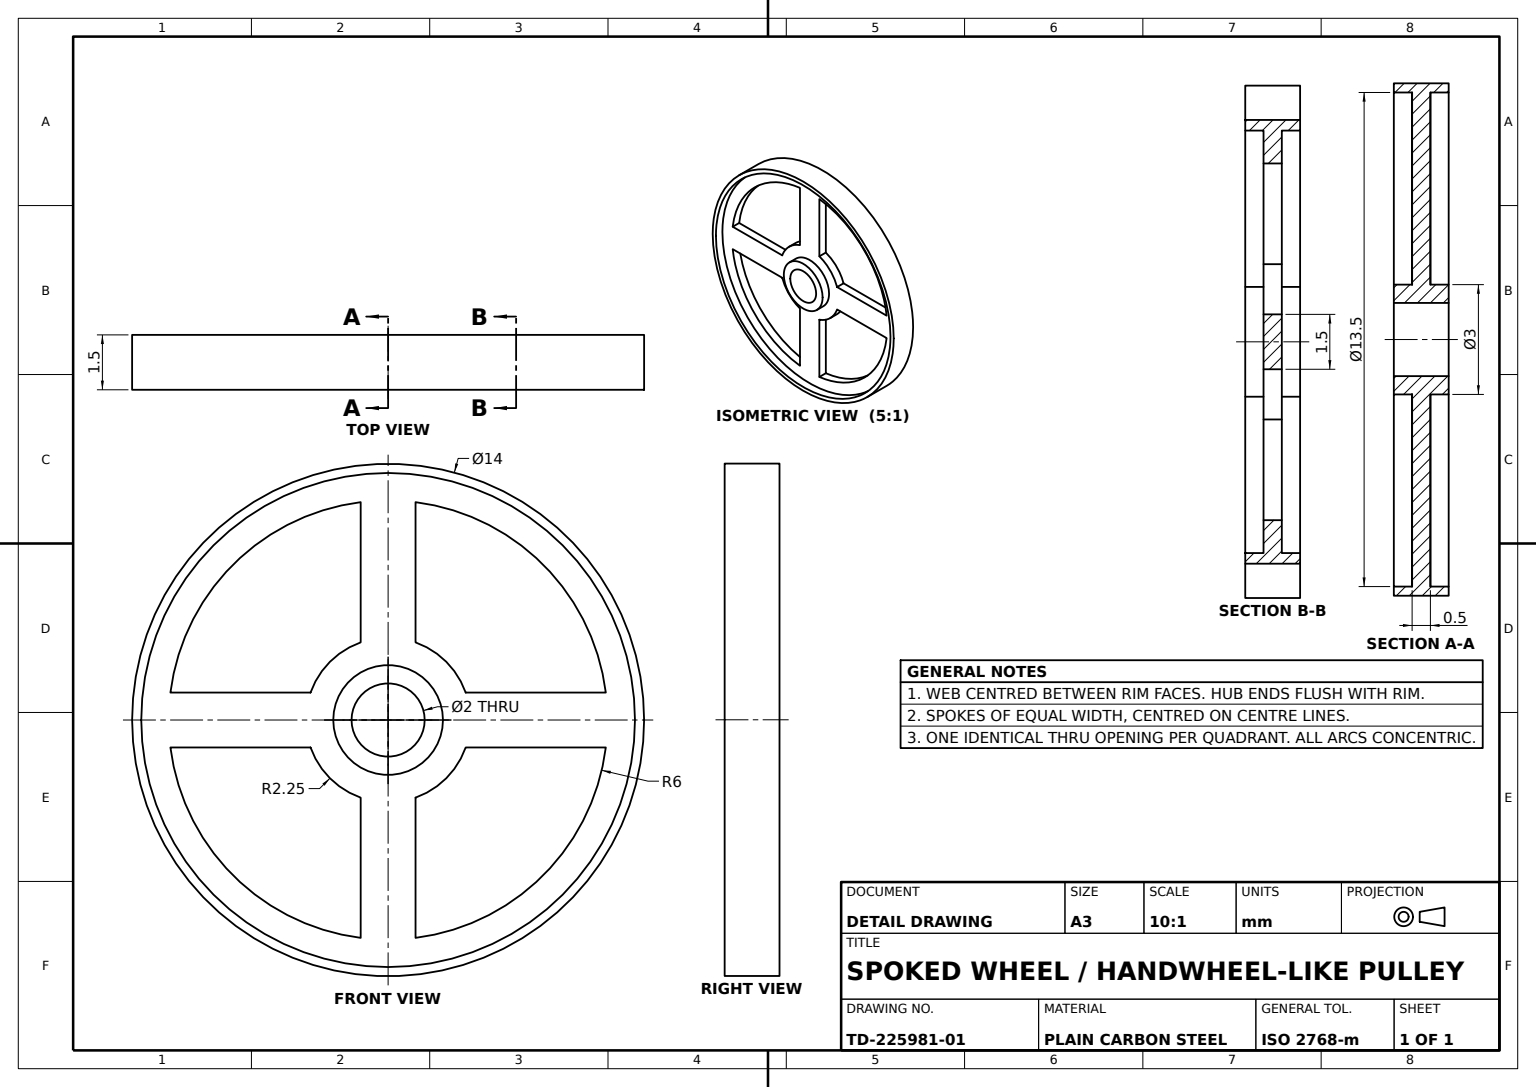
SolidWorks part; units mm, degrees
material "Plain Carbon Steel"
ref_plane "Front Plane" through (0, 0, 0) normal (0, 0, 1) x (1, 0, 0)
ref_plane "Top Plane" through (0, 0, 0) normal (0, 1, 0) x (1, 0, 0)
ref_plane "Right Plane" through (0, 0, 0) normal (1, 0, 0) x (0, 0, -1)
sketch "Hub Core Sketch" plane through (0, 0, 0) normal (0, 0, 1) x (1, 0, 0)
  circle A0 centre (0, 0) radius 2.25
  dimension "D1" = 2.25
extrude "Hub Core" add sketch "Hub Core Sketch" along normal blind 0.5
sketch "Hub Flange Sketch" plane through (0, 0, 0.5) normal (0, 0, 1) x (1, 0, 0)
  circle A0 centre (0, 0) radius 6
  dimension "D1" = 6
extrude "Hub Flange Ø6" add sketch "Hub Flange Sketch" along normal blind 0.5
sketch "Front Hub Boss Sketch" plane through (0, 0, 1) normal (0, 0, 1) x (1, 0, 0)
  circle A0 centre (0, 0) radius 2.25
  dimension "D1" = 2.25
extrude "Front Hub Boss" add sketch "Front Hub Boss Sketch" along normal blind 0.5
sketch "Cross Slot Sketch" plane through (0, 0, 1) normal (0, 0, 1) x (1, 0, 0)
  line L0 (0, 0) -> (0.75, 0)
  line L1 (0.75, 0) -> (0.75, 6.4066)
  line L2 (0.75, 6.4066) -> (-0.75, 6.4066)
  line L3 (-0.75, 6.4066) -> (-0.75, -6.4896)
  line L4 (-0.75, -6.4896) -> (0.75, -6.4896)
  line L5 (0.75, -6.4896) -> (0.75, 0)
  line L6 (0, 0) -> (0, 0.75)
  line L7 (0, 0.75) -> (8.267, 0.75)
  line L8 (8.267, 0.75) -> (8.267, -0.75)
  line L9 (8.267, -0.75) -> (-7.6768, -0.75)
  line L10 (-7.6768, -0.75) -> (-7.6768, 0.75)
  line L11 (-7.6768, 0.75) -> (0, 0.75)
  circle M1 centre (0, 0) radius 2.25
  circle M2 centre (0, 0) radius 6
  dimension "D1" = 0.75
  dimension "D2" = 1.5
  dimension "D3" = 1.5
  dimension "D4" = 0.75
  dimension "D5" = 1.5
  dimension "D6" = 1.5
  dimension "D7" = 6.4066
  dimension "D8" = 6.4896
  dimension "D9" = 8.267
  dimension "D10" = 7.6768
extrude "Cross Slot Cut" cut sketch "Cross Slot Sketch" against normal blind 0.5 contours L11 L3 M2 M1 | L7 L1 M1 M2 | L9 L5 M2 M1 | L9 L3 M1 M2
sketch "Web Ring Sketch" plane through (0, 0, 1) normal (0, 0, 1) x (1, 0, 0)
  circle A0 centre (0, 0) radius 6.75
  circle A1 centre (0, 0) radius 6
  dimension "D1" = 13.5
  dimension "D2" = 6
extrude "Web Ring Ø13.5" add sketch "Web Ring Sketch" against normal blind 0.5
sketch "Front Hub Hole Sketch" plane through (0, 0, 1.5) normal (0, 0, 1) x (1, 0, 0)
  circle A0 centre (0, 0) radius 2.25
  dimension "D1" = 4.5
extrude "Front Hub Hole Cut" cut sketch "Front Hub Hole Sketch" against normal blind 0.5
sketch "Back Hub Recess Sketch" plane through (0, 0, 0) normal (0, 0, -1) x (-1, 0, 0)
  circle A0 centre (0, 0) radius 2.25
  dimension "D1" = 4.5
extrude "Back Hub Recess Cut" cut sketch "Back Hub Recess Sketch" against normal blind 0.5
sketch "Hub Ring A Sketch" plane through (0, 0, 0.5) normal (0, 0, -1) x (-1, 0, 0)
  circle A0 centre (0, 0) radius 1.5
  dimension "D1" = 3
extrude "Hub Ring A" add sketch "Hub Ring A Sketch" along normal blind 0.5
sketch "Hub Ring B Sketch" plane through (0, 0, 1) normal (0, 0, 1) x (1, 0, 0)
  circle A0 centre (0, 0) radius 1.5
  dimension "D1" = 3
extrude "Hub Ring B" add sketch "Hub Ring B Sketch" along normal blind 0.5
sketch "Spoke 1 Sketch" plane through (0, -0.75, 0) normal (0, -1, 0) x (1, 0, 0)
  line L0 (-1.5, 1.5) -> (-1.5, 1)
  line L1 (-1.5, 1) -> (-6.75, 1)
  line L2 (6.75, 1) -> (-6.75, 1) construction
  line L3 (-1.5, 1.5) -> (-5.25, 1.5)
  line L5 (-5.25, 1.5) -> (-6.75, 1)
  dimension "D1" = 1.5
  dimension "D2" = 5.25
extrude "Spoke 1" add sketch "Spoke 1 Sketch" against normal blind 1.5 separate body
sketch "Spoke 1 Groove A Sketch" plane through (0, -0.75, 0) normal (0, -1, 0) x (1, 0, 0)
  line L0 (-6.75, 1) -> (-5.25, 1.5)
  line L1 (-5.25, 1.5) -> (-1.5, 1.5)
  line L2 (-1.5, 1.5) -> (-1.5, 1)
  line L3 (-1.5, 1) -> (-6.75, 1)
extrude "Spoke 1 Groove A" cut sketch "Spoke 1 Groove A Sketch" against normal blind 0.625
sketch "Spoke 1 Groove B Sketch" plane through (0, 0.75, 0) normal (0, 1, 0) x (1, 0, 0)
  line L0 (-1.5, -1.5) -> (-1.5, -1)
  line L1 (-1.5, -1) -> (-6.75, -1)
  line L2 (-6.75, -1) -> (-5.25, -1.5)
  line L3 (-5.25, -1.5) -> (-1.5, -1.5)
extrude "Spoke 1 Groove B" cut sketch "Spoke 1 Groove B Sketch" against normal blind 0.625
sketch "Spoke 2 Sketch" plane through (0, -0.75, 0) normal (0, -1, 0) x (1, 0, 0)
  line L0 (1.5, 1.5) -> (1.5, 1)
  line L1 (1.5, 1) -> (6.75, 1)
  line L2 (0, 1.5) -> (5.25, 1.5)
  line L3 (1.5, 1.5) -> (-1.5, 1.5) construction
  line L4 (5.25, 1.5) -> (6.75, 1)
  line M1 (5.9529, 1) -> (2.1213, 1)
  dimension "D1" = 5.25
extrude "Spoke 2" add sketch "Spoke 2 Sketch" against normal blind 1.5 separate body contours L4 L2 L0 L1 M1
sketch "Spoke 3 Sketch" plane through (0, -0.75, 0) normal (0, -1, 0) x (1, 0, 0)
  line L0 (1.5, 0) -> (1.5, 0.5)
  line L1 (1.5, 0.5) -> (6.75, 0.5)
  line L2 (1.5, 0) -> (5.25, 0)
  line L3 (5.25, 0) -> (6.75, 0.5)
  dimension "D1" = 1.5
extrude "Spoke 3" add sketch "Spoke 3 Sketch" against normal blind 1.5 separate body
sketch "Spoke 4 Sketch" plane through (0, -0.75, 0) normal (0, -1, 0) x (1, 0, 0)
  line L0 (-1.5, 0) -> (-5.25, 0)
  line L1 (-6.75, 0.5) -> (-5.25, 0)
  line L2 (-6.75, 0.5) -> (-1.5, 0.5)
  line L3 (-1.5, 0.5) -> (-1.5, 0)
  line L4 (-1.5, 0.5) -> (-1.5, 0) construction
  dimension "D1" = 3.75
  dimension "D2" = 0.5
extrude "Spoke 4" add sketch "Spoke 4 Sketch" against normal blind 1.5 separate body
sketch "Spoke Grooves A Sketch" plane through (0, -0.75, 0) normal (0, -1, 0) x (1, 0, 0)
  line L0 (1.5, 1.5) -> (1.5, 1)
  line L1 (1.5, 1) -> (6.75, 1)
  line L2 (6.75, 1) -> (5.25, 1.5)
  line L3 (5.25, 1.5) -> (1.5, 1.5)
  line L4 (1.5, 0) -> (1.5, 0.5)
  line L5 (1.5, 0.5) -> (6.75, 0.5)
  line L6 (6.75, 0.5) -> (5.25, 0)
  line L7 (5.25, 0) -> (1.5, 0)
  line L8 (-6.75, 0.5) -> (-1.5, 0.5)
  line L9 (-1.5, 0.5) -> (-1.5, 0)
  line L10 (-1.5, 0) -> (-5.25, 0)
  line L11 (-5.25, 0) -> (-6.75, 0.5)
extrude "Spoke Grooves A" cut sketch "Spoke Grooves A Sketch" against normal blind 0.65
sketch "Spoke Grooves B Sketch" plane through (0, 0.75, 0) normal (0, 1, 0) x (1, 0, 0)
  line L0 (1.5, 0) -> (5.25, 0)
  line L1 (5.25, 0) -> (6.75, -0.5)
  line L2 (6.75, -0.5) -> (1.5, -0.5)
  line L3 (1.5, -0.5) -> (1.5, 0)
  line L4 (1.5, -1.5) -> (1.5, -1)
  line L5 (1.5, -1.5) -> (1.5, -1) construction
  line L6 (1.5, -1) -> (6.75, -1)
  line L7 (6.75, -1) -> (5.25, -1.5)
  line L8 (5.25, -1.5) -> (1.5, -1.5)
  line L9 (-6.75, -0.5) -> (-1.5, -0.5)
  line L10 (-1.5, -0.5) -> (-1.5, 0)
  line L11 (-1.5, 0) -> (-5.25, 0)
  line L12 (-5.25, 0) -> (-6.75, -0.5)
extrude "Spoke Grooves B" cut sketch "Spoke Grooves B Sketch" against normal blind 0.65
sketch "Cross Spokes Sketch" plane through (-0.75, 0, 0) normal (-1, 0, 0) x (0, 0, 1)
  line L0 (1, 1.5) -> (1, 6.75)
  line L1 (0.5, 1.5) -> (0.5, 6.75)
  line L2 (1.5, 1.5) -> (1.5, 5.25)
  line L4 (1.5, 5.25) -> (1, 6.75)
  line L5 (0, 1.5) -> (0, 5.25)
  line L6 (0, 5.25) -> (0.5, 6.75)
  line L7 (1, -1.5) -> (1, -6.75)
  line L8 (1.5, -1.5) -> (1.5, -5.25)
  line L9 (1.5, -5.25) -> (1, -6.75)
  line L10 (0.5, -1.5) -> (0.5, -6.75)
  line L11 (0, -1.5) -> (0, -5.25)
  line L12 (0, -5.25) -> (0.5, -6.75)
  line L13 (0.5, 1.5) -> (0, 1.5)
  line L14 (0.5, 1.5) -> (0, 1.5) construction
  line L15 (1, 1.5) -> (1.5, 1.5)
  line L16 (1.5, 1.5) -> (1, 1.5) construction
  line L17 (1, -1.5) -> (1.5, -1.5)
  line L18 (0.5, -1.5) -> (0, -1.5)
  line L19 (0, -1.5) -> (0.5, -1.5) construction
  dimension "D1" = 0.5
  dimension "D2" = 0.5
  dimension "D3" = 1.5
  dimension "D4" = 1.5
  dimension "D5" = 3.75
  dimension "D6" = 5.25
  dimension "D7" = 1.5811
  dimension "D8" = 3.75
  dimension "D9" = 0.5
extrude "Cross Spokes" add sketch "Cross Spokes Sketch" against normal blind 1.5 separate body
sketch "Cross Spoke Grooves A Sketch" plane through (-0.75, 0, 0) normal (-1, 0, 0) x (0, 0, 1)
  line L0 (1.5, 1.5) -> (1, 1.5)
  line L1 (1, 1.5) -> (1, 6.75)
  line L2 (1, 6.75) -> (1.5, 5.25)
  line L3 (1.5, 5.25) -> (1.5, 1.5)
  line L4 (0.5, 6.75) -> (0.5, 1.5)
  line L5 (0.5, 1.5) -> (0, 1.5)
  line L6 (0, 1.5) -> (0, 5.25)
  line L7 (0, 5.25) -> (0.5, 6.75)
  line L8 (1, -6.75) -> (1, -1.5)
  line L9 (1, -1.5) -> (1.5, -1.5)
  line L10 (1.5, -1.5) -> (1.5, -5.25)
  line L11 (1.5, -5.25) -> (1, -6.75)
  line L12 (0, -1.5) -> (0.5, -1.5)
  line L13 (0.5, -1.5) -> (0.5, -6.75)
  line L14 (0.5, -6.75) -> (0, -5.25)
  line L15 (0, -5.25) -> (0, -1.5)
extrude "Cross Spoke Grooves A" cut sketch "Cross Spoke Grooves A Sketch" against normal blind 0.625
sketch "Cross Spoke Grooves B Sketch" plane through (0.75, 0, 0) normal (1, 0, 0) x (0, 0, -1)
  line L0 (0, 1.5) -> (-0.5, 1.5)
  line L1 (-0.5, 1.5) -> (-0.5, 6.75)
  line L2 (-0.5, 6.75) -> (0, 5.25)
  line L3 (0, 5.25) -> (0, 1.5)
  line L4 (-1, 6.75) -> (-1, 1.5)
  line L5 (-1, 1.5) -> (-1.5, 1.5)
  line L6 (-1.5, 1.5) -> (-1.5, 5.25)
  line L7 (-1.5, 5.25) -> (-1, 6.75)
  line L8 (0, -1.5) -> (0, -5.25)
  line L9 (0, -5.25) -> (-0.5, -6.75)
  line L10 (-0.5, -6.75) -> (-0.5, -1.5)
  line L11 (-0.5, -1.5) -> (0, -1.5)
  line L12 (-1.5, -1.5) -> (-1.5, -5.25)
  line L13 (-1.5, -5.25) -> (-1, -6.75)
  line L14 (-1, -6.75) -> (-1, -1.5)
  line L15 (-1, -1.5) -> (-1.5, -1.5)
extrude "Cross Spoke Grooves B" cut sketch "Cross Spoke Grooves B Sketch" against normal blind 0.625
sketch "Centre Hole Sketch" plane through (0, 0, 1.5) normal (0, 0, 1) x (1, 0, 0)
  circle A0 centre (0, 0) radius 1
  dimension "D1" = 2
extrude "Centre Hole Cut" cut sketch "Centre Hole Sketch" against normal blind 10
sketch "Rim Ring 1 Sketch" plane through (0, 0, 1) normal (0, 0, 1) x (1, 0, 0)
  circle A0 centre (0, 0) radius 7
  circle A1 centre (0, 0) radius 6.75
  dimension "D1" = 14
  dimension "D2" = 13.5
extrude "Rim Ring 1 Ø14" add sketch "Rim Ring 1 Sketch" against normal blind 0.5
sketch "Rim Ring 2 Sketch" plane through (0, 0, 1) normal (0, 0, 1) x (1, 0, 0)
  circle A0 centre (0, 0) radius 7
  circle A1 centre (0, 0) radius 6.75
  dimension "D1" = 14
  dimension "D2" = 13.5
extrude "Rim Ring 2 Ø14" add sketch "Rim Ring 2 Sketch" along normal blind 0.5
sketch "Rim Ring 3 Sketch" plane through (0, 0, 0.5) normal (0, 0, -1) x (-1, 0, 0)
  circle A0 centre (0, 0) radius 7
  circle A1 centre (0, 0) radius 6.75
  dimension "D1" = 13.5
  dimension "D2" = 14
extrude "Rim Ring 3 Ø14" add sketch "Rim Ring 3 Sketch" along normal blind 0.5
delete or keep bodies "Body-Delete/Keep 1" type delete bodies bodies 134 120 122 132 113 121 131 133
